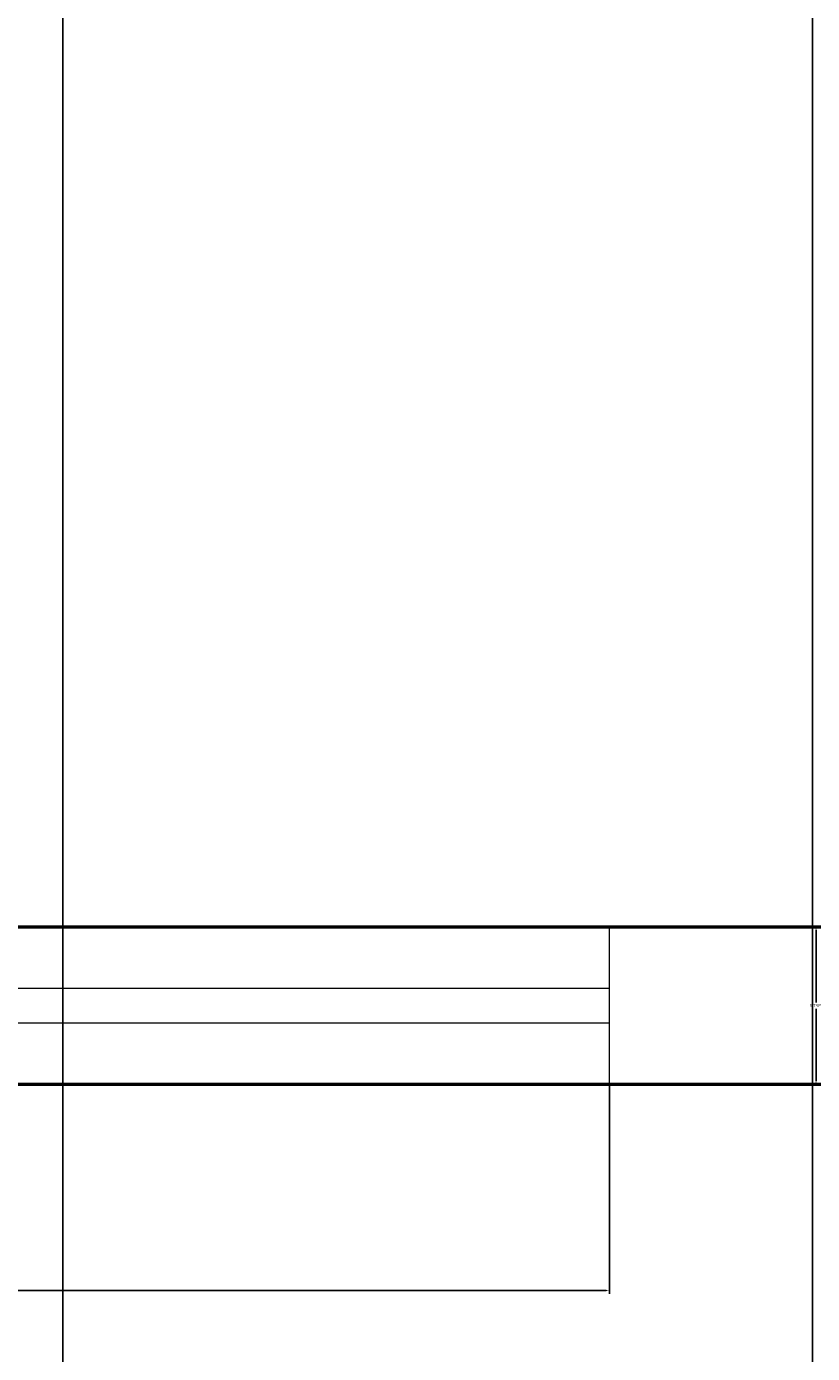
# Model space of a CAD drawing. Units: inches. Extents: x 7359 to 7979, y 33027 to 34263.
# Tile 25 of 32: x 7597 to 7641, y 33749 to 33825. Entities that reach past the tile are written whole.
import ezdxf

# ---------------------------------------------------------------- set-up
doc = ezdxf.new("R2010")
doc.units = ezdxf.units.IN
for name, color, linetype, lineweight in [('A-ANNO-DIMS', 2, 'Continuous', 18), ('A-GLAZ', 4, 'Continuous', 18), ('A-WALL', 7, 'Continuous', 50)]:
    doc.layers.add(name, color=color, linetype=linetype, lineweight=lineweight)
doc.styles.get("Standard").update_dxf_attribs({"font": 'arial.ttf'})
doc.dimstyles.get("Standard").update_dxf_attribs({"dimtxt": 0.18, "dimasz": 0.18, "dimexe": 0.18, "dimexo": 0.0625, "dimgap": 0.09, "dimtad": 0, "dimtih": 1, "dimtoh": 1, "dimdec": 4, "dimzin": 0, "dimdsep": 46, "dimtxsty": 'Standard', "dimcen": 0.09, "dimadec": 0, "dimazin": 0, "dimtfac": 1, "dimtdec": 4, "dimtofl": 0, "dimtmove": 0, "dimatfit": 3, "dimfxl": 1, "dimtolj": 1, "dimtzin": 0, "dimarcsym": 0})

# ---------------------------------------------------------------- blocks, each defined once
blk = doc.blocks.new('WINDOW-W1-DRAWING-FRONT')
for p, q in [((0, 0), (0, 9)), ((78.794, 0), (78.794, 9)), ((0, 5.5), (78.794, 5.5)), ((0, 3.5), (78.794, 3.5))]:
    blk.add_line(p, q)
blk = doc.blocks.new('*D62')
at = {"layer": 'A-ANNO-DIMS', "color": 0, "lineweight": -2, "transparency": 16777216}
for p, q in [((7551.084, 33764.771), (7551.084, 33752.835)), ((7629.878, 33764.771), (7629.878, 33752.835)), ((7551.264, 33753.015), (7589.266, 33753.015)), ((7629.698, 33753.015), (7591.695, 33753.015))]:
    blk.add_line(p, q, dxfattribs=at)
at = {"layer": 'A-ANNO-DIMS', "color": 0, "transparency": 16777216}
for points in [[(7551.264, 33753.045), (7551.264, 33752.985), (7551.084, 33753.015)], [(7629.698, 33753.045), (7629.698, 33752.985), (7629.878, 33753.015)]]:
    blk.add_solid(points, dxfattribs=at)
at = {"layer": 'Defpoints', "color": 0, "transparency": 16777216}
for p in [(7551.084, 33764.834), (7629.878, 33764.834), (7629.878, 33753.015)]:
    blk.add_point(p, dxfattribs=at)
at = {"layer": 'A-ANNO-DIMS', "color": 0, "transparency": 16777216, "insert": (7590.481, 33753.015), "char_height": 0.18, "attachment_point": 5}
blk.add_mtext('\\A1;FRONT W1 79 TYP.', dxfattribs=at)
blk = doc.blocks.new('*D63')
at = {"layer": 'A-ANNO-DIMS', "color": 0, "lineweight": -2, "transparency": 16777216}
for p, q in [((7629.94, 33773.834), (7641.877, 33773.834)), ((7641.697, 33773.654), (7641.697, 33769.516)), ((7641.697, 33765.014), (7641.697, 33769.152)), ((7629.94, 33764.834), (7641.877, 33764.834))]:
    blk.add_line(p, q, dxfattribs=at)
at = {"layer": 'A-ANNO-DIMS', "color": 0, "transparency": 16777216}
for points in [[(7641.667, 33773.654), (7641.727, 33773.654), (7641.697, 33773.834)], [(7641.667, 33765.014), (7641.727, 33765.014), (7641.697, 33764.834)]]:
    blk.add_solid(points, dxfattribs=at)
at = {"layer": 'Defpoints', "color": 0, "transparency": 16777216}
for p in [(7629.878, 33773.834), (7641.697, 33773.834), (7629.878, 33764.834)]:
    blk.add_point(p, dxfattribs=at)
at = {"layer": 'A-ANNO-DIMS', "color": 0, "transparency": 16777216, "insert": (7641.697, 33769.334), "char_height": 0.18, "attachment_point": 5}
blk.add_mtext('\\A1;9 TYP.', dxfattribs=at)
blk = doc.blocks.new('*D71')
at = {"layer": 'A-ANNO-DIMS', "color": 0, "lineweight": -2, "transparency": 16777216}
for p, q in [((7641.491, 33907.171), (7641.491, 33632.309)), ((7683.491, 33907.171), (7683.491, 33632.309)), ((7641.671, 33632.489), (7662.27, 33632.489)), ((7683.311, 33632.489), (7662.713, 33632.489))]:
    blk.add_line(p, q, dxfattribs=at)
at = {"layer": 'A-ANNO-DIMS', "color": 0, "transparency": 16777216}
for points in [[(7641.671, 33632.519), (7641.671, 33632.459), (7641.491, 33632.489)], [(7683.311, 33632.519), (7683.311, 33632.459), (7683.491, 33632.489)]]:
    blk.add_solid(points, dxfattribs=at)
at = {"layer": 'Defpoints', "color": 0, "transparency": 16777216}
for p in [(7641.491, 33907.234), (7683.491, 33907.234), (7683.491, 33632.489)]:
    blk.add_point(p, dxfattribs=at)
at = {"layer": 'A-ANNO-DIMS', "color": 0, "transparency": 16777216, "insert": (7662.491, 33632.489), "char_height": 0.18, "attachment_point": 5}
blk.add_mtext('\\A1;42', dxfattribs=at)
blk = doc.blocks.new('*D83')
at = {"layer": 'A-ANNO-DIMS', "color": 0, "lineweight": -2, "transparency": 16777216}
for p, q in [((7592.591484, 34081.771428), (7592.591484, 33632.309146)), ((7598.591484, 34081.771428), (7598.591484, 33632.309146)), ((7592.771484, 33632.489146), (7595.442057, 33632.489146)), ((7598.411484, 33632.489146), (7595.740911, 33632.489146))]:
    blk.add_line(p, q, dxfattribs=at)
at = {"layer": 'A-ANNO-DIMS', "color": 0, "transparency": 16777216}
for points in [[(7592.771484, 33632.519146), (7592.771484, 33632.459146), (7592.591484, 33632.489146)], [(7598.411484, 33632.519146), (7598.411484, 33632.459146), (7598.591484, 33632.489146)]]:
    blk.add_solid(points, dxfattribs=at)
at = {"layer": 'Defpoints', "color": 0, "transparency": 16777216}
for p in [(7592.591484, 34081.833928), (7598.591484, 34081.833928), (7598.591484, 33632.489146)]:
    blk.add_point(p, dxfattribs=at)
at = {"layer": 'A-ANNO-DIMS', "color": 0, "transparency": 16777216, "insert": (7595.591484, 33632.489146), "char_height": 0.18, "attachment_point": 5}
blk.add_mtext('\\A1;6', dxfattribs=at)

msp = doc.modelspace()

# ---------------------------------------------------------------- linework, layer by layer
at = {"layer": 'A-WALL'}
for p, q in [((7467.5915, 33773.8339), (7689.4915, 33773.8339)), ((7458.5915, 33764.8339), (7883.9915, 33764.8339))]:
    msp.add_line(p, q, dxfattribs=at)

# ---------------------------------------------------------------- block references
at = {"layer": 'A-GLAZ'}
msp.add_blockref('WINDOW-W1-DRAWING-FRONT', (7551.084, 33764.834), dxfattribs=at)

# ---------------------------------------------------------------- dimensions: what is measured, and where the dimension line sits
at = {"layer": 'A-ANNO-DIMS'}
for base, p1, p2, picture, middle in [((7598.5915, 33632.4891), (7592.5915, 34081.8339), (7598.5915, 34081.8339), '*D83', (7595.5915, 33632.4891)), ((7683.4915, 33632.4891), (7641.4915, 33907.2339), (7683.4915, 33907.2339), '*D71', (7662.4915, 33632.4891))]:
    dim = msp.add_linear_dim(base=base, p1=p1, p2=p2, dimstyle='Standard', override={"dimdec": 0, "dimlfac": 1, "dimrnd": 0, "dimzin": 0, "dimdsep": 46, "dimlunit": 2}, dxfattribs=at)
    dim.commit()
    dim.dimension.update_dxf_attribs({"geometry": picture, "text_midpoint": middle})
dim = msp.add_linear_dim(base=(7641.6969, 33773.8339), p1=(7629.8778, 33764.8339), p2=(7629.8778, 33773.8339), angle=90, text='<> TYP.', dimstyle='Standard', override={"dimdec": 0, "dimlfac": 1, "dimrnd": 0, "dimzin": 0, "dimdsep": 46, "dimlunit": 2}, dxfattribs=at)
dim.commit()
dim.dimension.update_dxf_attribs({"geometry": '*D63', "text_midpoint": (7641.6969, 33769.3339)})
dim = msp.add_linear_dim(base=(7629.8778, 33753.0149), p1=(7551.0841, 33764.8339), p2=(7629.8778, 33764.8339), text='FRONT W1 <> TYP.', dimstyle='Standard', override={"dimdec": 0, "dimlfac": 1, "dimrnd": 0, "dimzin": 0, "dimdsep": 46, "dimlunit": 2}, dxfattribs=at)
dim.commit()
dim.dimension.update_dxf_attribs({"geometry": '*D62', "text_midpoint": (7590.4809, 33753.0149)})

doc.saveas('drawing.dxf')
